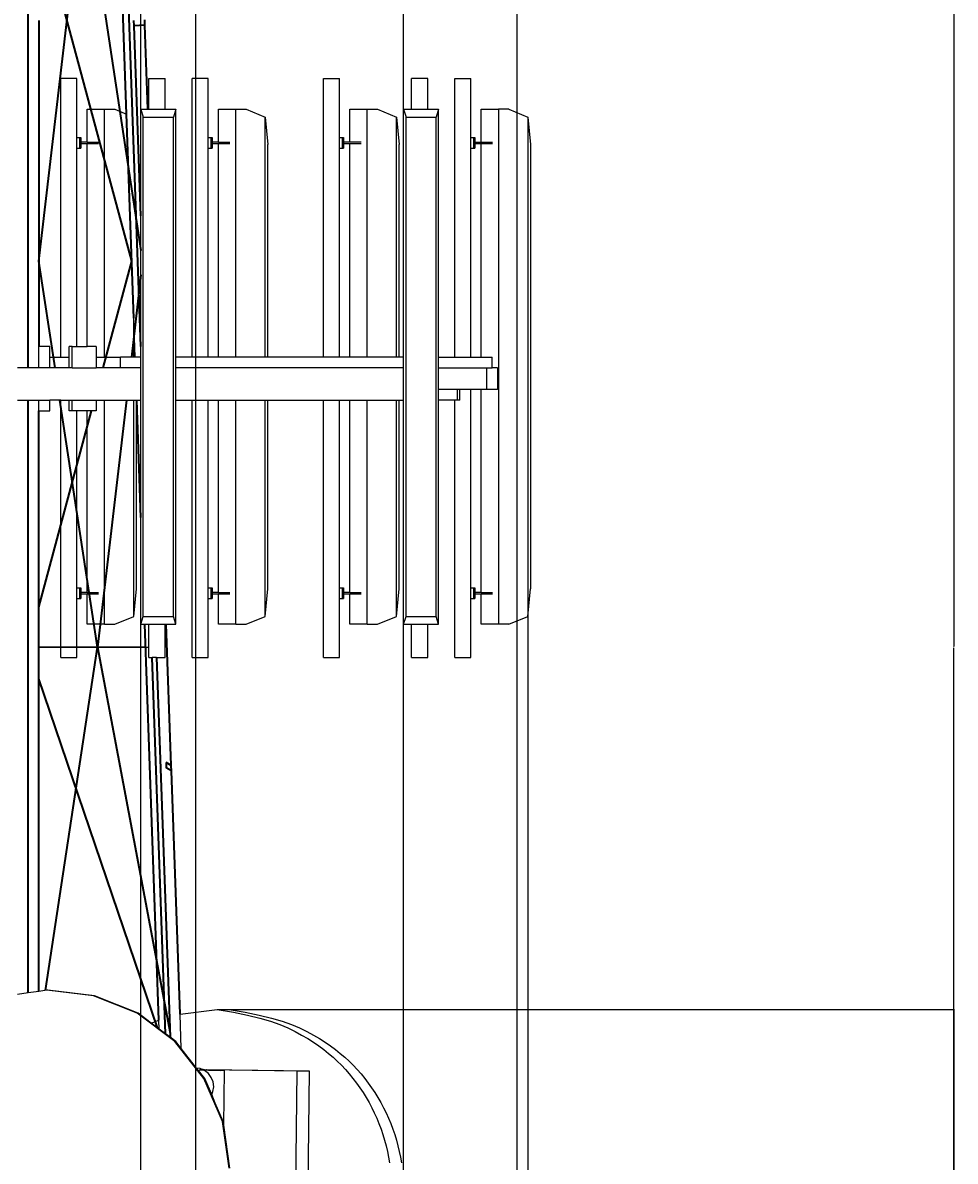
# Model space of a CAD drawing. Units: inches. Extents: x 3780 to 4301, y 1637 to 4224.
# Tile 7 of 8: x 4040 to 4301, y 3542 to 3860. Entities that reach past the tile are written whole.
import ezdxf

# ---------------------------------------------------------------- set-up
doc = ezdxf.new("R2010")
doc.units = ezdxf.units.IN
for name, color, linetype, lineweight in [('A-ANNO-DIMS', 2, 'Continuous', 18), ('E-COMM-ANTN', 4, 'Continuous', 25), ('E-COMM-DISH', 3, 'Continuous', 25), ('S-TOWR', 7, 'Continuous', 35)]:
    doc.layers.add(name, color=color, linetype=linetype, lineweight=lineweight)
doc.styles.get("Standard").update_dxf_attribs({"font": 'arial.ttf'})
doc.dimstyles.get("Standard").update_dxf_attribs({"dimtxt": 0.18, "dimasz": 0.18, "dimexe": 0.18, "dimexo": 0.0625, "dimgap": 0.09, "dimtad": 0, "dimtih": 1, "dimtoh": 1, "dimdec": 4, "dimzin": 0, "dimdsep": 46, "dimtxsty": 'Standard', "dimcen": 0.09, "dimadec": 0, "dimazin": 0, "dimtfac": 1, "dimtdec": 4, "dimtofl": 0, "dimtmove": 0, "dimatfit": 3, "dimfxl": 1, "dimtolj": 1, "dimtzin": 0, "dimarcsym": 0})

# ---------------------------------------------------------------- blocks, each defined once
blk = doc.blocks.new('ANT-PANEL')
for p, q in [((3905.38, 3835.91), (3900.05, 3833.75)), ((3905.38, 3835.91), (3908.22, 3835.91)), ((3908.22, 3691.91), (3908.22, 3835.91)), ((3900.05, 3833.75), (3899.34, 3826.07)), ((3900.05, 3694.07), (3900.05, 3833.75)), ((3899.34, 3701.75), (3899.34, 3826.07)), ((3900.05, 3694.07), (3899.34, 3701.75)), ((3905.38, 3691.91), (3900.05, 3694.07)), ((3905.38, 3691.91), (3908.22, 3691.91))]:
    blk.add_line(p, q)
blk = doc.blocks.new('ANT-PANEL-MOUNT-B')
for p, q in [((4148.97, 3835.91), (4148.97, 3844.56)), ((4153.47, 3844.56), (4148.97, 3844.56)), ((4153.47, 3835.91), (4153.47, 3844.56)), ((4146.73, 3835.91), (4147.4, 3833.75)), ((4146.73, 3835.91), (4148.97, 3835.91)), ((4146.73, 3766.56), (4146.73, 3835.91)), ((4148.97, 3835.91), (4153.47, 3835.91)), ((4153.47, 3835.91), (4156.48, 3835.91)), ((4156.48, 3835.91), (4155.82, 3833.75)), ((4156.48, 3766.56), (4156.48, 3835.91)), ((4147.4, 3833.75), (4155.82, 3833.75)), ((4147.4, 3694.07), (4147.4, 3833.75)), ((4155.82, 3694.07), (4155.82, 3833.75)), ((4146.73, 3763.56), (4146.73, 3766.56)), ((4156.48, 3763.56), (4156.48, 3766.56)), ((4146.73, 3754.56), (4146.73, 3763.56)), ((4156.48, 3757.56), (4156.48, 3763.56)), ((4156.48, 3754.56), (4156.48, 3757.56)), ((4146.73, 3691.91), (4146.73, 3754.56)), ((4156.48, 3691.91), (4156.48, 3754.56)), ((4146.73, 3691.91), (4147.4, 3694.07)), ((4146.73, 3691.91), (4148.97, 3691.91)), ((4147.4, 3694.07), (4155.82, 3694.07)), ((4148.97, 3682.56), (4148.97, 3691.91)), ((4148.97, 3691.91), (4153.47, 3691.91)), ((4153.47, 3682.56), (4153.47, 3691.91)), ((4153.47, 3691.91), (4156.48, 3691.91)), ((4156.48, 3691.91), (4155.82, 3694.07)), ((4148.97, 3682.56), (4153.47, 3682.56))]:
    blk.add_line(p, q)
blk = doc.blocks.new('*D21')
at = {"layer": 'A-ANNO-DIMS', "color": 0, "lineweight": -2, "transparency": 16777216}
for p, q in [((4010.55, 3901.46), (4300.89, 3901.46)), ((4300.71, 3901.28), (4300.71, 3685.65)), ((4300.71, 3469.64), (4300.71, 3685.28)), ((4044.72, 3469.46), (4300.89, 3469.46))]:
    blk.add_line(p, q, dxfattribs=at)
at = {"layer": 'A-ANNO-DIMS', "color": 0, "transparency": 16777216}
for points in [[(4300.68, 3901.28), (4300.74, 3901.28), (4300.71, 3901.46)], [(4300.68, 3469.64), (4300.74, 3469.64), (4300.71, 3469.46)]]:
    blk.add_solid(points, dxfattribs=at)
at = {"layer": 'Defpoints', "color": 0, "transparency": 16777216}
for p in [(4010.49, 3901.46), (4300.71, 3901.46), (4044.66, 3469.46)]:
    blk.add_point(p, dxfattribs=at)
at = {"layer": 'A-ANNO-DIMS', "color": 0, "transparency": 16777216, "insert": (4300.71, 3685.46), "char_height": 0.18, "attachment_point": 5}
blk.add_mtext('\\A1;432', dxfattribs=at)
blk = doc.blocks.new('*D22')
at = {"layer": 'A-ANNO-DIMS', "color": 0, "lineweight": -2, "transparency": 16777216}
for p, q in [((3900.05, 3694.01), (3900.05, 1636.57)), ((4181.5, 3694.01), (4181.5, 1636.57)), ((3900.23, 1636.75), (4040.31, 1636.75)), ((4181.32, 1636.75), (4041.24, 1636.75))]:
    blk.add_line(p, q, dxfattribs=at)
at = {"layer": 'A-ANNO-DIMS', "color": 0, "transparency": 16777216}
for points in [[(3900.23, 1636.78), (3900.23, 1636.72), (3900.05, 1636.75)], [(4181.32, 1636.78), (4181.32, 1636.72), (4181.5, 1636.75)]]:
    blk.add_solid(points, dxfattribs=at)
at = {"layer": 'Defpoints', "color": 0, "transparency": 16777216}
for p in [(3900.05, 3694.07), (4181.5, 3694.07), (4181.5, 1636.75)]:
    blk.add_point(p, dxfattribs=at)
at = {"layer": 'A-ANNO-DIMS', "color": 0, "transparency": 16777216, "insert": (4040.77, 1636.75), "char_height": 0.18, "attachment_point": 5}
blk.add_mtext('\\A1;281.45', dxfattribs=at)
blk = doc.blocks.new('*D28')
at = {"layer": 'A-ANNO-DIMS', "color": 0, "lineweight": -2, "transparency": 16777216}
for p, q in [((3926.17, 3691.91), (3780.66, 3691.91)), ((3780.84, 3691.73), (3780.84, 3590.48)), ((3780.84, 3488.87), (3780.84, 3590.12)), ((4048.31, 3488.69), (3780.66, 3488.69))]:
    blk.add_line(p, q, dxfattribs=at)
at = {"layer": 'A-ANNO-DIMS', "color": 0, "transparency": 16777216}
for points in [[(3780.81, 3691.73), (3780.87, 3691.73), (3780.84, 3691.91)], [(3780.81, 3488.87), (3780.87, 3488.87), (3780.84, 3488.69)]]:
    blk.add_solid(points, dxfattribs=at)
at = {"layer": 'Defpoints', "color": 0, "transparency": 16777216}
for p in [(3780.84, 3691.91), (3926.23, 3691.91), (4048.37, 3488.69)]:
    blk.add_point(p, dxfattribs=at)
at = {"layer": 'A-ANNO-DIMS', "color": 0, "transparency": 16777216, "insert": (3780.84, 3590.3), "char_height": 0.18, "attachment_point": 5}
blk.add_mtext('\\A1;203.2', dxfattribs=at)
blk = doc.blocks.new('*D40')
at = {"layer": 'A-ANNO-DIMS', "color": 0, "lineweight": -2, "transparency": 16777216}
for p, q in [((3999.73, 3835.97), (3999.73, 4223.96)), ((3999.91, 4223.78), (4036.16, 4223.78)), ((4073.05, 4223.78), (4036.81, 4223.78)), ((4073.23, 3835.97), (4073.23, 4223.96))]:
    blk.add_line(p, q, dxfattribs=at)
at = {"layer": 'A-ANNO-DIMS', "color": 0, "transparency": 16777216}
for points in [[(3999.91, 4223.81), (3999.91, 4223.75), (3999.73, 4223.78)], [(4073.05, 4223.81), (4073.05, 4223.75), (4073.23, 4223.78)]]:
    blk.add_solid(points, dxfattribs=at)
at = {"layer": 'Defpoints', "color": 0, "transparency": 16777216}
for p in [(4073.23, 4223.78), (3999.73, 3835.91), (4073.23, 3835.91)]:
    blk.add_point(p, dxfattribs=at)
at = {"layer": 'A-ANNO-DIMS', "color": 0, "transparency": 16777216, "insert": (4036.48, 4223.78), "char_height": 0.18, "attachment_point": 5}
blk.add_mtext('\\A1;73.5', dxfattribs=at)
blk = doc.blocks.new('*D41')
at = {"layer": 'A-ANNO-DIMS', "color": 0, "lineweight": -2, "transparency": 16777216}
for p, q in [((4073.23, 3835.97), (4073.23, 4223.96)), ((4073.41, 4223.78), (4109.66, 4223.78)), ((4146.55, 4223.78), (4110.31, 4223.78)), ((4146.73, 3835.97), (4146.73, 4223.96))]:
    blk.add_line(p, q, dxfattribs=at)
at = {"layer": 'A-ANNO-DIMS', "color": 0, "transparency": 16777216}
for points in [[(4073.41, 4223.81), (4073.41, 4223.75), (4073.23, 4223.78)], [(4146.55, 4223.81), (4146.55, 4223.75), (4146.73, 4223.78)]]:
    blk.add_solid(points, dxfattribs=at)
at = {"layer": 'Defpoints', "color": 0, "transparency": 16777216}
for p in [(4146.73, 4223.78), (4073.23, 3835.91), (4146.73, 3835.91)]:
    blk.add_point(p, dxfattribs=at)
at = {"layer": 'A-ANNO-DIMS', "color": 0, "transparency": 16777216, "insert": (4109.98, 4223.78), "char_height": 0.18, "attachment_point": 5}
blk.add_mtext('\\A1;73.5', dxfattribs=at)
blk = doc.blocks.new('*D45')
at = {"layer": 'A-ANNO-DIMS', "color": 0, "lineweight": -2, "transparency": 16777216}
for p, q in [((3971.79, 3552.9), (3780.66, 3552.9)), ((3780.84, 3552.72), (3780.84, 3520.98)), ((3780.84, 3488.87), (3780.84, 3520.61)), ((4048.31, 3488.69), (3780.66, 3488.69))]:
    blk.add_line(p, q, dxfattribs=at)
at = {"layer": 'A-ANNO-DIMS', "color": 0, "transparency": 16777216}
for points in [[(3780.81, 3552.72), (3780.87, 3552.72), (3780.84, 3552.9)], [(3780.81, 3488.87), (3780.87, 3488.87), (3780.84, 3488.69)]]:
    blk.add_solid(points, dxfattribs=at)
at = {"layer": 'Defpoints', "color": 0, "transparency": 16777216}
for p in [(3780.84, 3552.9), (3971.85, 3552.9), (4048.37, 3488.69)]:
    blk.add_point(p, dxfattribs=at)
at = {"layer": 'A-ANNO-DIMS', "color": 0, "transparency": 16777216, "insert": (3780.84, 3520.8), "char_height": 0.18, "attachment_point": 5}
blk.add_mtext('\\A1;64.21', dxfattribs=at)
blk = doc.blocks.new('*D47')
at = {"layer": 'A-ANNO-DIMS', "color": 0, "lineweight": -2, "transparency": 16777216}
for p, q in [((4094.64, 3584.08), (4300.89, 3584.08)), ((4300.71, 3583.9), (4300.71, 3533.86)), ((4300.71, 3483.47), (4300.71, 3533.5)), ((4093.42, 3483.29), (4300.89, 3483.29))]:
    blk.add_line(p, q, dxfattribs=at)
at = {"layer": 'A-ANNO-DIMS', "color": 0, "transparency": 16777216}
for points in [[(4300.68, 3583.9), (4300.74, 3583.9), (4300.71, 3584.08)], [(4300.68, 3483.47), (4300.74, 3483.47), (4300.71, 3483.29)]]:
    blk.add_solid(points, dxfattribs=at)
at = {"layer": 'Defpoints', "color": 0, "transparency": 16777216}
for p in [(4094.58, 3584.08), (4093.36, 3483.29), (4300.71, 3483.29)]:
    blk.add_point(p, dxfattribs=at)
at = {"layer": 'A-ANNO-DIMS', "color": 0, "transparency": 16777216, "insert": (4300.71, 3533.68), "char_height": 0.18, "attachment_point": 5}
blk.add_mtext('\\A1;100.79', dxfattribs=at)
blk = doc.blocks.new('*D49')
at = {"layer": 'A-ANNO-DIMS', "color": 0, "lineweight": -2, "transparency": 16777216}
for p, q in [((3999.73, 3245.63), (3999.73, 4223.96)), ((3999.91, 4223.78), (4036.16, 4223.78)), ((4073.05, 4223.78), (4036.81, 4223.78)), ((4073.23, 3245.63), (4073.23, 4223.96))]:
    blk.add_line(p, q, dxfattribs=at)
at = {"layer": 'A-ANNO-DIMS', "color": 0, "transparency": 16777216}
for points in [[(3999.91, 4223.81), (3999.91, 4223.75), (3999.73, 4223.78)], [(4073.05, 4223.81), (4073.05, 4223.75), (4073.23, 4223.78)]]:
    blk.add_solid(points, dxfattribs=at)
at = {"layer": 'Defpoints', "color": 0, "transparency": 16777216}
for p in [(4073.23, 4223.78), (3999.73, 3245.56), (4073.23, 3245.56)]:
    blk.add_point(p, dxfattribs=at)
at = {"layer": 'A-ANNO-DIMS', "color": 0, "transparency": 16777216, "insert": (4036.48, 4223.78), "char_height": 0.18, "attachment_point": 5}
blk.add_mtext('\\A1;73.5', dxfattribs=at)
blk = doc.blocks.new('*D50')
at = {"layer": 'A-ANNO-DIMS', "color": 0, "lineweight": -2, "transparency": 16777216}
for p, q in [((4073.23, 3245.63), (4073.23, 4223.96)), ((4073.41, 4223.78), (4109.66, 4223.78)), ((4146.55, 4223.78), (4110.31, 4223.78)), ((4146.73, 3245.63), (4146.73, 4223.96))]:
    blk.add_line(p, q, dxfattribs=at)
at = {"layer": 'A-ANNO-DIMS', "color": 0, "transparency": 16777216}
for points in [[(4073.41, 4223.81), (4073.41, 4223.75), (4073.23, 4223.78)], [(4146.55, 4223.81), (4146.55, 4223.75), (4146.73, 4223.78)]]:
    blk.add_solid(points, dxfattribs=at)
at = {"layer": 'Defpoints', "color": 0, "transparency": 16777216}
for p in [(4146.73, 4223.78), (4073.23, 3245.56), (4146.73, 3245.56)]:
    blk.add_point(p, dxfattribs=at)
at = {"layer": 'A-ANNO-DIMS', "color": 0, "transparency": 16777216, "insert": (4109.98, 4223.78), "char_height": 0.18, "attachment_point": 5}
blk.add_mtext('\\A1;73.5', dxfattribs=at)
blk = doc.blocks.new('*D59')
at = {"layer": 'A-ANNO-DIMS', "color": 0, "lineweight": -2, "transparency": 16777216}
for p, q in [((4088.55, 3352.58), (4088.55, 4223.96)), ((4088.73, 4223.78), (4133.13, 4223.78)), ((4178.28, 4223.78), (4133.88, 4223.78)), ((4178.46, 3329.55), (4178.46, 4223.96))]:
    blk.add_line(p, q, dxfattribs=at)
at = {"layer": 'A-ANNO-DIMS', "color": 0, "transparency": 16777216}
for points in [[(4088.73, 4223.81), (4088.73, 4223.75), (4088.55, 4223.78)], [(4178.28, 4223.81), (4178.28, 4223.75), (4178.46, 4223.78)]]:
    blk.add_solid(points, dxfattribs=at)
at = {"layer": 'Defpoints', "color": 0, "transparency": 16777216}
for p in [(4178.46, 4223.78), (4088.55, 3352.51), (4178.46, 3329.49)]:
    blk.add_point(p, dxfattribs=at)
at = {"layer": 'A-ANNO-DIMS', "color": 0, "transparency": 16777216, "insert": (4133.51, 4223.78), "char_height": 0.18, "attachment_point": 5}
blk.add_mtext('\\A1;89.91', dxfattribs=at)

msp = doc.modelspace()

# ---------------------------------------------------------------- linework, layer by layer
at = {"layer": 'E-COMM-ANTN'}
for p, q in [((4050.7911, 3766.5582), (4050.7911, 3844.5582)), ((4055.2911, 3844.5582), (4050.7911, 3844.5582)), ((4055.2911, 3828.0582), (4055.2911, 3844.5582)), ((4075.4676, 3835.9077), (4075.4676, 3844.5582)), ((4075.4676, 3844.5582), (4079.9676, 3844.5582)), ((4079.9676, 3835.9077), (4079.9676, 3844.5582)), ((4087.5411, 3766.5582), (4087.5411, 3844.5582)), ((4092.0411, 3844.5582), (4087.5411, 3844.5582)), ((4092.0411, 3828.0582), (4092.0411, 3844.5582)), ((4124.2911, 3766.5582), (4124.2911, 3844.5582)), ((4124.2911, 3844.5582), (4128.7911, 3844.5582)), ((4128.7911, 3828.0582), (4128.7911, 3844.5582)), ((4161.0411, 3766.5582), (4161.0411, 3844.5582)), ((4161.0411, 3844.5582), (4165.5411, 3844.5582)), ((4165.5411, 3828.0582), (4165.5411, 3844.5582)), ((4058.2034, 3826.7457), (4058.2034, 3835.9077)), ((4058.2034, 3835.9077), (4063.0784, 3835.9077)), ((4063.0784, 3835.9077), (4065.9127, 3835.9077)), ((4063.0784, 3766.5582), (4063.0784, 3835.9077)), ((4065.9127, 3835.9077), (4069.2183, 3834.5694)), ((4073.2315, 3835.9077), (4073.8979, 3833.7477)), ((4073.2315, 3835.9077), (4075.1707, 3835.9077)), ((4073.2315, 3806.0827), (4073.2315, 3835.9077)), ((4075.1707, 3835.9077), (4075.4676, 3835.9077)), ((4075.4676, 3835.9077), (4079.9676, 3835.9077)), ((4079.9676, 3835.9077), (4082.9815, 3835.9077)), ((4082.9815, 3835.9077), (4082.3151, 3833.7477)), ((4082.9815, 3766.5582), (4082.9815, 3835.9077)), ((4094.9534, 3826.7457), (4094.9534, 3835.9077)), ((4094.9534, 3835.9077), (4099.8284, 3835.9077)), ((4099.8284, 3835.9077), (4102.6627, 3835.9077)), ((4099.8284, 3766.5582), (4099.8284, 3835.9077)), ((4102.6627, 3835.9077), (4107.998, 3833.7477)), ((4131.7034, 3826.7457), (4131.7034, 3835.9077)), ((4131.7034, 3835.9077), (4136.5784, 3835.9077)), ((4136.5784, 3835.9077), (4139.4127, 3835.9077)), ((4136.5784, 3766.5582), (4136.5784, 3835.9077)), ((4139.4127, 3835.9077), (4144.748, 3833.7477)), ((4168.4534, 3826.7457), (4168.4534, 3835.9077)), ((4168.4534, 3835.9077), (4173.3284, 3835.9077)), ((4073.8979, 3833.7477), (4082.3151, 3833.7477)), ((4073.8979, 3694.0677), (4073.8979, 3833.7477)), ((4082.3151, 3694.0677), (4082.3151, 3833.7477)), ((4107.998, 3766.5582), (4107.998, 3833.7477)), ((4107.998, 3833.7477), (4108.7091, 3826.0653)), ((4144.748, 3833.7477), (4145.4591, 3826.0653)), ((4144.748, 3766.5582), (4144.748, 3833.7477)), ((4055.2911, 3828.0582), (4056.1147, 3828.0582)), ((4055.2911, 3825.0582), (4055.2911, 3828.0582)), ((4056.1147, 3828.0582), (4056.4394, 3828.0582)), ((4056.1147, 3825.0582), (4056.1147, 3828.0582)), ((4056.4394, 3828.0582), (4056.4394, 3826.7457)), ((4092.0411, 3828.0582), (4092.8647, 3828.0582)), ((4092.0411, 3825.0582), (4092.0411, 3828.0582)), ((4092.8647, 3828.0582), (4093.1894, 3828.0582)), ((4092.8647, 3825.0582), (4092.8647, 3828.0582)), ((4093.1894, 3828.0582), (4093.1894, 3826.7457)), ((4128.7911, 3828.0582), (4129.6147, 3828.0582)), ((4128.7911, 3825.0582), (4128.7911, 3828.0582)), ((4129.6147, 3825.0582), (4129.6147, 3828.0582)), ((4129.6147, 3828.0582), (4129.9394, 3828.0582)), ((4129.9394, 3828.0582), (4129.9394, 3826.7457)), ((4165.5411, 3828.0582), (4166.3647, 3828.0582)), ((4165.5411, 3825.0582), (4165.5411, 3828.0582)), ((4166.3647, 3828.0582), (4166.6894, 3828.0582)), ((4166.3647, 3825.0582), (4166.3647, 3828.0582)), ((4166.6894, 3828.0582), (4166.6894, 3826.7457)), ((4055.2911, 3825.0582), (4056.1147, 3825.0582)), ((4055.2911, 3769.5582), (4055.2911, 3825.0582)), ((4056.1147, 3825.0582), (4056.4394, 3825.0582)), ((4058.2034, 3826.7457), (4056.4394, 3826.7457)), ((4056.4394, 3826.7457), (4056.4394, 3826.3707)), ((4056.4394, 3826.3707), (4056.4394, 3825.0582)), ((4056.4394, 3826.3707), (4058.2034, 3826.3707)), ((4058.2034, 3826.7457), (4061.3979, 3826.7457)), ((4058.2034, 3769.5582), (4058.2034, 3826.3707)), ((4058.2034, 3826.3707), (4061.3979, 3826.3707)), ((4092.0411, 3825.0582), (4092.8647, 3825.0582)), ((4092.0411, 3766.5582), (4092.0411, 3825.0582)), ((4092.8647, 3825.0582), (4093.1894, 3825.0582)), ((4094.9534, 3826.7457), (4093.1894, 3826.7457)), ((4093.1894, 3826.7457), (4093.1894, 3826.3707)), ((4093.1894, 3826.3707), (4094.9534, 3826.3707)), ((4093.1894, 3826.3707), (4093.1894, 3825.0582)), ((4094.9534, 3826.7457), (4098.1479, 3826.7457)), ((4094.9534, 3766.5582), (4094.9534, 3826.3707)), ((4094.9534, 3826.3707), (4098.1479, 3826.3707)), ((4108.7091, 3766.5582), (4108.7091, 3826.0653)), ((4128.7911, 3825.0582), (4129.6147, 3825.0582)), ((4128.7911, 3766.5582), (4128.7911, 3825.0582)), ((4129.6147, 3825.0582), (4129.9394, 3825.0582)), ((4131.7034, 3826.7457), (4129.9394, 3826.7457)), ((4129.9394, 3826.7457), (4129.9394, 3826.3707)), ((4129.9394, 3826.3707), (4131.7034, 3826.3707)), ((4129.9394, 3826.3707), (4129.9394, 3825.0582)), ((4134.8979, 3826.7457), (4131.7034, 3826.7457)), ((4131.7034, 3766.5582), (4131.7034, 3826.3707)), ((4131.7034, 3826.3707), (4134.8979, 3826.3707)), ((4145.4591, 3766.5582), (4145.4591, 3826.0653)), ((4165.5411, 3825.0582), (4166.3647, 3825.0582)), ((4165.5411, 3766.5582), (4165.5411, 3825.0582)), ((4166.3647, 3825.0582), (4166.6894, 3825.0582)), ((4166.6894, 3826.7457), (4168.4534, 3826.7457)), ((4166.6894, 3826.7457), (4166.6894, 3826.3707)), ((4166.6894, 3826.3707), (4168.4534, 3826.3707)), ((4166.6894, 3826.3707), (4166.6894, 3825.0582)), ((4168.4534, 3826.7457), (4171.6479, 3826.7457)), ((4168.4534, 3766.5582), (4168.4534, 3826.3707)), ((4168.4534, 3826.3707), (4171.6479, 3826.3707)), ((4073.2315, 3769.5583), (4073.2315, 3806.0827)), ((4071.248, 3766.5582), (4071.248, 3777.502)), ((4071.6372, 3766.5582), (4071.248, 3777.502)), ((4047.7176, 3769.5582), (4044.6622, 3769.5582)), ((4044.6622, 3763.5582), (4044.6622, 3769.5582)), ((4047.7176, 3766.5582), (4047.7176, 3769.5582)), ((4053.9472, 3769.5582), (4053.181, 3769.5582)), ((4053.181, 3766.5582), (4053.181, 3769.5582)), ((4053.9472, 3763.5582), (4053.9472, 3769.5582)), ((4053.9472, 3769.5582), (4055.2911, 3769.5582)), ((4055.2911, 3769.5582), (4058.2034, 3769.5582)), ((4060.6972, 3769.5582), (4058.2034, 3769.5582)), ((4060.6972, 3769.5582), (4060.6972, 3766.5582)), ((4073.2315, 3766.5582), (4073.2315, 3769.5583)), ((4047.7176, 3763.5582), (4047.7176, 3766.5582)), ((4047.7176, 3766.5582), (4050.7911, 3766.5582)), ((4050.7911, 3766.5582), (4053.181, 3766.5582)), ((4053.181, 3763.5582), (4053.181, 3766.5582)), ((4060.6972, 3766.5582), (4060.6972, 3763.5582)), ((4060.6972, 3766.5582), (4063.0784, 3766.5582)), ((4063.0784, 3766.5582), (4067.5445, 3766.5582)), ((4067.5445, 3763.5582), (4067.5445, 3766.5582)), ((4071.248, 3766.5582), (4067.5445, 3766.5582)), ((4071.6372, 3766.5582), (4071.248, 3766.5582)), ((4073.2315, 3766.5582), (4071.6372, 3766.5582)), ((4073.2315, 3763.5582), (4073.2315, 3766.5582)), ((4087.5411, 3766.5582), (4082.9815, 3766.5582)), ((4082.9815, 3763.5582), (4082.9815, 3766.5582)), ((4092.0411, 3766.5582), (4087.5411, 3766.5582)), ((4094.9534, 3766.5582), (4092.0411, 3766.5582)), ((4099.8284, 3766.5582), (4094.9534, 3766.5582)), ((4107.998, 3766.5582), (4099.8284, 3766.5582)), ((4108.7091, 3766.5582), (4107.998, 3766.5582)), ((4124.2911, 3766.5582), (4108.7091, 3766.5582)), ((4128.7911, 3766.5582), (4124.2911, 3766.5582)), ((4131.7034, 3766.5582), (4128.7911, 3766.5582)), ((4136.5784, 3766.5582), (4131.7034, 3766.5582)), ((4144.748, 3766.5582), (4136.5784, 3766.5582)), ((4145.4591, 3766.5582), (4144.748, 3766.5582)), ((4146.7315, 3766.5582), (4145.4591, 3766.5582)), ((4156.4815, 3766.5582), (4161.0411, 3766.5582)), ((4161.0411, 3766.5582), (4165.5411, 3766.5582)), ((4165.5411, 3766.5582), (4168.4534, 3766.5582)), ((4168.4534, 3766.5582), (4171.4676, 3766.5582)), ((4171.4676, 3763.5582), (4171.4676, 3766.5582)), ((4041.6622, 3763.5582), (4038.6622, 3763.5582)), ((4044.6622, 3763.5582), (4041.6622, 3763.5582)), ((4047.7176, 3763.5582), (4044.6622, 3763.5582)), ((4053.181, 3763.5582), (4047.7176, 3763.5582)), ((4053.9472, 3763.5582), (4053.181, 3763.5582)), ((4053.9472, 3763.5582), (4060.6972, 3763.5582)), ((4067.5445, 3763.5582), (4060.6972, 3763.5582)), ((4073.2315, 3763.5582), (4067.5445, 3763.5582)), ((4073.2315, 3754.5582), (4073.2315, 3763.5582)), ((4146.7315, 3763.5582), (4082.9815, 3763.5582)), ((4082.9815, 3754.5582), (4082.9815, 3763.5582)), ((4156.4815, 3763.5582), (4169.976, 3763.5582)), ((4169.976, 3763.5582), (4171.4676, 3763.5582)), ((4169.976, 3757.5582), (4169.976, 3763.5582)), ((4172.9591, 3763.5582), (4171.4676, 3763.5582)), ((4172.9591, 3763.5582), (4172.9591, 3757.5582)), ((4161.818, 3757.5582), (4156.4815, 3757.5582)), ((4161.818, 3754.5582), (4161.818, 3757.5582)), ((4162.4676, 3757.5582), (4161.818, 3757.5582)), ((4162.4676, 3754.5582), (4162.4676, 3757.5582)), ((4165.5411, 3757.5582), (4162.4676, 3757.5582)), ((4165.5411, 3702.0582), (4165.5411, 3757.5582)), ((4168.4534, 3757.5582), (4165.5411, 3757.5582)), ((4168.4534, 3700.7457), (4168.4534, 3757.5582)), ((4169.976, 3757.5582), (4168.4534, 3757.5582)), ((4172.9591, 3757.5582), (4169.976, 3757.5582)), ((4038.6622, 3754.5582), (4041.6622, 3754.5582)), ((4041.6622, 3754.5582), (4044.6622, 3754.5582)), ((4044.6622, 3751.5582), (4044.6622, 3754.5582)), ((4044.6622, 3754.5582), (4047.7176, 3754.5582)), ((4044.6622, 3751.5582), (4047.7176, 3751.5582)), ((4047.7176, 3751.5582), (4047.7176, 3754.5582)), ((4050.7911, 3754.5582), (4047.7176, 3754.5582)), ((4050.7911, 3682.5582), (4050.7911, 3754.5582)), ((4050.7911, 3754.5582), (4053.181, 3754.5582)), ((4053.181, 3751.5582), (4053.181, 3754.5582)), ((4053.181, 3754.5582), (4053.9472, 3754.5582)), ((4053.9472, 3751.5582), (4053.181, 3751.5582)), ((4053.9472, 3751.5582), (4053.9472, 3754.5582)), ((4053.9472, 3754.5582), (4060.6972, 3754.5582)), ((4055.2911, 3751.5582), (4053.9472, 3751.5582)), ((4058.2034, 3751.5582), (4055.2911, 3751.5582)), ((4055.2911, 3702.0582), (4055.2911, 3751.5582)), ((4058.2034, 3700.7457), (4058.2034, 3751.5582)), ((4060.6972, 3751.5582), (4058.2034, 3751.5582)), ((4060.6972, 3754.5582), (4060.6972, 3751.5582)), ((4060.6972, 3754.5582), (4063.0784, 3754.5582)), ((4063.0784, 3691.9077), (4063.0784, 3754.5582)), ((4063.0784, 3754.5582), (4071.248, 3754.5582)), ((4071.248, 3694.0677), (4071.248, 3754.5582)), ((4071.248, 3754.5582), (4071.9591, 3754.5582)), ((4071.9591, 3701.7501), (4071.9591, 3754.5582)), ((4071.9591, 3754.5582), (4072.064, 3754.5582)), ((4072.064, 3754.5582), (4073.2315, 3754.5582)), ((4073.2315, 3721.7331), (4073.2315, 3754.5582)), ((4082.9815, 3691.9077), (4082.9815, 3754.5582)), ((4082.9815, 3754.5582), (4087.5411, 3754.5582)), ((4087.5411, 3682.5582), (4087.5411, 3754.5582)), ((4087.5411, 3754.5582), (4092.0411, 3754.5582)), ((4092.0411, 3754.5582), (4094.9534, 3754.5582)), ((4092.0411, 3702.0582), (4092.0411, 3754.5582)), ((4094.9534, 3700.7457), (4094.9534, 3754.5582)), ((4094.9534, 3754.5582), (4099.8284, 3754.5582)), ((4099.8284, 3691.9077), (4099.8284, 3754.5582)), ((4099.8284, 3754.5582), (4107.998, 3754.5582)), ((4107.998, 3694.0677), (4107.998, 3754.5582)), ((4107.998, 3754.5582), (4108.7091, 3754.5582)), ((4108.7091, 3701.7501), (4108.7091, 3754.5582)), ((4108.7091, 3754.5582), (4124.2911, 3754.5582)), ((4124.2911, 3682.5582), (4124.2911, 3754.5582)), ((4124.2911, 3754.5582), (4128.7911, 3754.5582)), ((4128.7911, 3702.0582), (4128.7911, 3754.5582)), ((4128.7911, 3754.5582), (4131.7034, 3754.5582)), ((4131.7034, 3700.7457), (4131.7034, 3754.5582)), ((4131.7034, 3754.5582), (4136.5784, 3754.5582)), ((4136.5784, 3691.9077), (4136.5784, 3754.5582)), ((4136.5784, 3754.5582), (4144.748, 3754.5582)), ((4144.748, 3694.0677), (4144.748, 3754.5582)), ((4144.748, 3754.5582), (4145.4591, 3754.5582)), ((4145.4591, 3701.7501), (4145.4591, 3754.5582)), ((4145.4591, 3754.5582), (4146.7315, 3754.5582)), ((4161.0411, 3754.5582), (4156.4815, 3754.5582)), ((4161.0411, 3682.5582), (4161.0411, 3754.5582)), ((4161.818, 3754.5582), (4161.0411, 3754.5582)), ((4162.4676, 3754.5582), (4161.818, 3754.5582)), ((4073.2315, 3691.9077), (4073.2315, 3721.7331)), ((4055.2911, 3702.0582), (4056.1147, 3702.0582)), ((4055.2911, 3699.0582), (4055.2911, 3702.0582)), ((4056.1147, 3699.0582), (4056.1147, 3702.0582)), ((4056.1147, 3702.0582), (4056.4394, 3702.0582)), ((4056.4394, 3702.0582), (4056.4394, 3700.7457)), ((4058.2034, 3700.7457), (4056.4394, 3700.7457)), ((4056.4394, 3700.7457), (4056.4394, 3700.3707)), ((4058.2034, 3700.7457), (4061.3979, 3700.7457)), ((4071.248, 3694.0677), (4071.9591, 3701.7501)), ((4092.0411, 3702.0582), (4092.8647, 3702.0582)), ((4092.0411, 3699.0582), (4092.0411, 3702.0582)), ((4092.8647, 3702.0582), (4093.1894, 3702.0582)), ((4092.8647, 3699.0582), (4092.8647, 3702.0582)), ((4093.1894, 3702.0582), (4093.1894, 3700.7457)), ((4094.9534, 3700.7457), (4093.1894, 3700.7457)), ((4093.1894, 3700.7457), (4093.1894, 3700.3707)), ((4094.9534, 3700.7457), (4098.1479, 3700.7457)), ((4107.998, 3694.0677), (4108.7091, 3701.7501)), ((4128.7911, 3702.0582), (4129.6147, 3702.0582)), ((4128.7911, 3699.0582), (4128.7911, 3702.0582)), ((4129.6147, 3699.0582), (4129.6147, 3702.0582)), ((4129.6147, 3702.0582), (4129.9394, 3702.0582)), ((4129.9394, 3702.0582), (4129.9394, 3700.7457)), ((4131.7034, 3700.7457), (4129.9394, 3700.7457)), ((4129.9394, 3700.7457), (4129.9394, 3700.3707)), ((4131.7034, 3700.7457), (4134.8979, 3700.7457)), ((4144.748, 3694.0677), (4145.4591, 3701.7501)), ((4165.5411, 3702.0582), (4166.3647, 3702.0582)), ((4165.5411, 3699.0582), (4165.5411, 3702.0582)), ((4166.3647, 3702.0582), (4166.6894, 3702.0582)), ((4166.3647, 3699.0582), (4166.3647, 3702.0582)), ((4166.6894, 3702.0582), (4166.6894, 3700.7457)), ((4168.4534, 3700.7457), (4166.6894, 3700.7457)), ((4166.6894, 3700.7457), (4166.6894, 3700.3707)), ((4168.4534, 3700.7457), (4171.6479, 3700.7457)), ((4055.2911, 3699.0582), (4056.1147, 3699.0582)), ((4055.2911, 3682.5582), (4055.2911, 3699.0582)), ((4056.1147, 3699.0582), (4056.4394, 3699.0582)), ((4056.4394, 3700.3707), (4056.4394, 3699.0582)), ((4056.4394, 3700.3707), (4058.2034, 3700.3707)), ((4058.2034, 3691.9077), (4058.2034, 3700.3707)), ((4058.2034, 3700.3707), (4061.3979, 3700.3707)), ((4092.0411, 3699.0582), (4092.8647, 3699.0582)), ((4092.0411, 3682.5582), (4092.0411, 3699.0582)), ((4092.8647, 3699.0582), (4093.1894, 3699.0582)), ((4093.1894, 3700.3707), (4094.9534, 3700.3707)), ((4093.1894, 3700.3707), (4093.1894, 3699.0582)), ((4094.9534, 3691.9077), (4094.9534, 3700.3707)), ((4094.9534, 3700.3707), (4098.1479, 3700.3707)), ((4128.7911, 3699.0582), (4129.6147, 3699.0582)), ((4128.7911, 3682.5582), (4128.7911, 3699.0582)), ((4129.6147, 3699.0582), (4129.9394, 3699.0582)), ((4129.9394, 3700.3707), (4129.9394, 3699.0582)), ((4129.9394, 3700.3707), (4131.7034, 3700.3707)), ((4131.7034, 3691.9077), (4131.7034, 3700.3707)), ((4131.7034, 3700.3707), (4134.8979, 3700.3707)), ((4165.5411, 3699.0582), (4166.3647, 3699.0582)), ((4165.5411, 3682.5582), (4165.5411, 3699.0582)), ((4166.3647, 3699.0582), (4166.6894, 3699.0582)), ((4166.6894, 3700.3707), (4168.4534, 3700.3707)), ((4166.6894, 3700.3707), (4166.6894, 3699.0582)), ((4168.4534, 3691.9077), (4168.4534, 3700.3707)), ((4168.4534, 3700.3707), (4171.6479, 3700.3707)), ((4063.0784, 3691.9077), (4058.2034, 3691.9077)), ((4063.0784, 3691.9077), (4065.9127, 3691.9077)), ((4065.9127, 3691.9077), (4071.248, 3694.0677)), ((4073.2315, 3691.9077), (4073.8979, 3694.0677)), ((4073.2315, 3691.9077), (4074.2923, 3691.9077)), ((4073.8979, 3694.0677), (4082.3151, 3694.0677)), ((4074.2923, 3691.9077), (4075.4676, 3691.9077)), ((4075.4676, 3682.5582), (4075.4676, 3691.9077)), ((4075.4676, 3691.9077), (4079.9676, 3691.9077)), ((4079.9676, 3682.5582), (4079.9676, 3691.9077)), ((4079.9676, 3691.9077), (4080.2923, 3691.9077)), ((4080.2923, 3691.9077), (4082.9815, 3691.9077)), ((4082.9815, 3691.9077), (4082.3151, 3694.0677)), ((4099.8284, 3691.9077), (4094.9534, 3691.9077)), ((4099.8284, 3691.9077), (4102.6627, 3691.9077)), ((4102.6627, 3691.9077), (4107.998, 3694.0677)), ((4136.5784, 3691.9077), (4131.7034, 3691.9077)), ((4136.5784, 3691.9077), (4139.4127, 3691.9077)), ((4139.4127, 3691.9077), (4144.748, 3694.0677)), ((4173.3284, 3691.9077), (4168.4534, 3691.9077)), ((4044.6622, 3685.4644), (4061.0918, 3685.4644)), ((4074.5214, 3685.4644), (4044.6622, 3685.4644)), ((4061.0918, 3685.4644), (4075.4676, 3685.4644)), ((4050.7911, 3682.5582), (4055.2911, 3682.5582)), ((4075.4676, 3682.5582), (4076.3257, 3682.5582)), ((4077.6248, 3682.5582), (4076.3257, 3682.5582)), ((4077.6248, 3682.5582), (4079.9676, 3682.5582)), ((4087.5411, 3682.5582), (4092.0411, 3682.5582)), ((4124.2911, 3682.5582), (4128.7911, 3682.5582)), ((4161.0411, 3682.5582), (4165.5411, 3682.5582))]:
    msp.add_line(p, q, dxfattribs=at)
at = {"layer": 'E-COMM-DISH'}
for p, q in [((4044.6622, 3589.1512), (4041.6622, 3588.7189)), ((4046.9214, 3589.4768), (4044.6622, 3589.1512)), ((4059.9847, 3587.919), (4046.9214, 3589.4768)), ((4047.1421, 3589.4768), (4046.9214, 3589.4768)), ((4060.2055, 3587.919), (4047.1421, 3589.4768)), ((4041.6622, 3588.7189), (4038.6622, 3588.2865)), ((4072.1998, 3583.0331), (4059.9847, 3587.919)), ((4072.4206, 3583.0331), (4060.2055, 3587.919)), ((4082.7342, 3575.1521), (4072.1998, 3583.0331)), ((4076.0934, 3580.2854), (4072.4206, 3583.0331)), ((4084.172, 3582.8241), (4094.5799, 3584.0758)), ((4084.5153, 3573.1691), (4084.172, 3582.8241)), ((4094.5799, 3584.0758), (4097.8821, 3584.0758)), ((4076.0934, 3580.2854), (4078.2316, 3581.1479)), ((4078.3215, 3578.6185), (4076.0934, 3580.2854)), ((4078.3215, 3578.6185), (4078.2316, 3581.1479)), ((4080.069, 3577.3112), (4078.3215, 3578.6185)), ((4081.4035, 3576.3128), (4080.069, 3577.3112)), ((4081.3626, 3577.4644), (4081.2095, 3576.4579)), ((4082.955, 3575.1521), (4081.4035, 3576.3128)), ((4090.8699, 3564.813), (4082.7342, 3575.1521)), ((4084.5153, 3573.1691), (4082.955, 3575.1521)), ((4088.808, 3567.714), (4084.5153, 3573.1691)), ((4089.7984, 3567.5719), (4088.808, 3567.714)), ((4089.338, 3567.0404), (4088.808, 3567.714)), ((4091.0907, 3564.813), (4089.338, 3567.0404)), ((4090.8854, 3567.1054), (4089.5444, 3567.1222)), ((4089.7984, 3567.5719), (4091.4395, 3567.2453)), ((4090.8598, 3567.1164), (4089.7984, 3567.5719)), ((4090.8598, 3567.1164), (4090.8494, 3567.1152)), ((4090.8598, 3567.1164), (4090.8854, 3567.1054)), ((4091.0455, 3567.0367), (4090.8854, 3567.1054)), ((4092.1116, 3566.1955), (4091.0455, 3567.0367)), ((4120.3822, 3566.8887), (4091.4395, 3567.2453)), ((4091.4395, 3567.2453), (4091.6644, 3567.2006)), ((4116.9751, 3566.8887), (4091.6644, 3567.2006)), ((4091.6644, 3567.2006), (4092.1732, 3567.0993)), ((4092.1732, 3567.0993), (4092.218, 3567.0893)), ((4092.218, 3567.0893), (4092.2229, 3567.0894)), ((4092.2229, 3567.0894), (4095.5689, 3567.0519)), ((4096.2502, 3567.0455), (4095.5689, 3567.0519)), ((4096.6029, 3567.0433), (4096.2502, 3567.0455)), ((4096.4173, 3551.7214), (4096.6029, 3567.0433)), ((4096.6029, 3567.0447), (4096.6029, 3567.0433)), ((4116.2249, 3504.9504), (4116.9751, 3566.8887)), ((4120.3822, 3566.8887), (4116.9751, 3566.8887)), ((4119.6319, 3504.9504), (4120.3822, 3566.8887)), ((4096.0526, 3552.7205), (4090.8699, 3564.813)), ((4093.03, 3560.288), (4091.0907, 3564.813)), ((4092.924, 3565.1054), (4092.1116, 3566.1955)), ((4093.4275, 3563.8409), (4092.924, 3565.1054)), ((4093.5876, 3562.4881), (4093.4275, 3563.8409)), ((4093.03, 3560.288), (4093.3935, 3561.1392)), ((4093.3935, 3561.1392), (4093.5876, 3562.4881)), ((4094.0364, 3557.9399), (4093.03, 3560.288)), ((4096.2734, 3552.7205), (4094.0364, 3557.9399)), ((4097.929, 3539.6986), (4096.0526, 3552.7205)), ((4096.4173, 3551.7214), (4096.2734, 3552.7205)), ((4098.1498, 3539.6986), (4096.4173, 3551.7214))]:
    msp.add_line(p, q, dxfattribs=at)
for points in [[(4094.5799, 3584.0758), (4099.1082, 3583.3399), (4103.054, 3582.5447), (4106.4833, 3581.6977), (4109.4621, 3580.8067), (4112.0563, 3579.8794), (4114.3318, 3578.9235), (4116.3546, 3577.9465), (4118.1907, 3576.9562), (4119.8966, 3575.9583), (4121.4921, 3574.9508), (4122.9874, 3573.9297), (4124.3929, 3572.891), (4125.719, 3571.8307), (4126.976, 3570.7449), (4128.1742, 3569.6295), (4129.324, 3568.4807), (4130.4338, 3567.2952), (4131.5044, 3566.0737), (4132.535, 3564.8175), (4133.5243, 3563.5281), (4134.4714, 3562.2067), (4135.3752, 3560.8549), (4136.2347, 3559.4741), (4137.0488, 3558.0656), (4137.8166, 3556.6308), (4138.5373, 3555.1714), (4139.2104, 3553.689), (4139.8351, 3552.1852), (4140.4109, 3550.6617), (4140.937, 3549.12), (4141.4129, 3547.5618), (4141.8378, 3545.9887), (4142.2113, 3544.4024), (4142.533, 3542.8046), (4142.8028, 3541.197)], [(4097.8821, 3584.0758), (4102.4104, 3583.3399), (4106.3562, 3582.5447), (4109.7855, 3581.6977), (4112.7643, 3580.8067), (4115.3585, 3579.8794), (4117.634, 3578.9235), (4119.6568, 3577.9465), (4121.4929, 3576.9562), (4123.1988, 3575.9583), (4124.7943, 3574.9508), (4126.2896, 3573.9297), (4127.6952, 3572.891), (4129.0212, 3571.8307), (4130.2782, 3570.7449), (4131.4764, 3569.6295), (4132.6262, 3568.4807), (4133.736, 3567.2952), (4134.8066, 3566.0737), (4135.8372, 3564.8175), (4136.8265, 3563.5281), (4137.7736, 3562.2067), (4138.6774, 3560.8549), (4139.5369, 3559.4741), (4140.351, 3558.0656), (4141.1188, 3556.6308), (4141.8396, 3555.1714), (4142.5126, 3553.689), (4143.1374, 3552.1852), (4143.7131, 3550.6617), (4144.2392, 3549.12), (4144.7151, 3547.5618), (4145.1401, 3545.9887), (4145.5135, 3544.4024), (4145.8352, 3542.8046), (4146.105, 3541.197)]]:
    msp.add_lwpolyline(points, dxfattribs=at)
at = {"layer": 'S-TOWR'}
for p, q in [((4041.6622, 3763.5582), (4041.6622, 3901.4644)), ((4044.6622, 3793.4644), (4057.2507, 3901.4644)), ((4070.6803, 3793.4644), (4044.6622, 3890.299)), ((4062.5275, 3866.7769), (4073.2315, 3796.4145)), ((4069.2183, 3834.5694), (4068.0728, 3866.7769)), ((4073.2315, 3769.5583), (4069.7738, 3866.7769)), ((4044.6622, 3860.7769), (4044.6622, 3769.5582)), ((4071.3402, 3859.2599), (4071.2869, 3860.7587)), ((4074.3326, 3859.473), (4074.2793, 3860.9717)), ((4074.3326, 3859.473), (4071.3402, 3859.2599)), ((4073.2315, 3806.0827), (4071.3402, 3859.2599)), ((4075.1707, 3835.9077), (4074.3326, 3859.473)), ((4071.248, 3777.502), (4069.2183, 3834.5694)), ((4049.2117, 3763.5582), (4044.6622, 3793.4644)), ((4062.6449, 3763.5582), (4070.6803, 3793.4644)), ((4073.2315, 3789.6141), (4070.5441, 3766.5582)), ((4041.6622, 3588.7189), (4041.6622, 3754.5582)), ((4044.6622, 3589.1512), (4044.6622, 3751.5582)), ((4044.6622, 3696.6299), (4059.4207, 3751.5582)), ((4061.0918, 3685.4644), (4050.5809, 3754.5582)), ((4069.1454, 3754.5582), (4061.0918, 3685.4644)), ((4073.2315, 3721.7331), (4072.064, 3754.5582)), ((4078.2316, 3581.1479), (4074.2923, 3691.9077)), ((4081.6998, 3652.3323), (4080.2923, 3691.9077)), ((4046.4799, 3589.4131), (4061.0918, 3685.4644)), ((4061.0918, 3685.4644), (4081.3626, 3577.4644)), ((4080.069, 3577.3112), (4076.3257, 3682.5582)), ((4077.6248, 3682.5582), (4081.4035, 3576.3128)), ((4077.8507, 3578.9707), (4044.6622, 3676.6362)), ((4081.6998, 3652.3323), (4080.2514, 3653.2216)), ((4080.2514, 3653.2216), (4080.3047, 3651.7228)), ((4081.7531, 3650.8336), (4080.3047, 3651.7228)), ((4081.7531, 3650.8336), (4081.6998, 3652.3323)), ((4084.172, 3582.8241), (4081.7531, 3650.8336))]:
    msp.add_line(p, q, dxfattribs=at)

# ---------------------------------------------------------------- block references
at = {"layer": 'E-COMM-ANTN'}
msp.add_blockref('ANT-PANEL-MOUNT-B', (0, 0), dxfattribs=at)
at = {"layer": 'E-COMM-ANTN', "rotation": 180}
msp.add_blockref('ANT-PANEL', (8081.5462, 7527.8153), dxfattribs=at)

# ---------------------------------------------------------------- dimensions: what is measured, and where the dimension line sits
at = {"layer": 'A-ANNO-DIMS'}
for base, p1, p2, override, picture, middle in [((4073.2315, 4223.7769), (3999.7315, 3835.9077), (4073.2315, 3835.9077), {"dimdec": 1, "dimlfac": 1, "dimrnd": 0, "dimzin": 0, "dimdsep": 46, "dimlunit": 2}, '*D40', (4036.4815, 4223.7769)), ((4073.2315, 4223.7769), (3999.7315, 3245.5639), (4073.2315, 3245.5639), {"dimdec": 1, "dimlfac": 1, "dimrnd": 0, "dimzin": 0, "dimdsep": 46, "dimlunit": 2}, '*D49', (4036.4815, 4223.7769)), ((4146.7315, 4223.7769), (4073.2315, 3835.9077), (4146.7315, 3835.9077), {"dimdec": 1, "dimlfac": 1, "dimrnd": 0, "dimzin": 0, "dimdsep": 46, "dimlunit": 2}, '*D41', (4109.9815, 4223.7769)), ((4146.7315, 4223.7769), (4073.2315, 3245.5639), (4146.7315, 3245.5639), {"dimdec": 1, "dimlfac": 1, "dimrnd": 0, "dimzin": 0, "dimdsep": 46, "dimlunit": 2}, '*D50', (4109.9815, 4223.7769)), ((4178.4631, 4223.7769), (4088.552, 3352.5141), (4178.4631, 3329.4859), {"dimdec": 2, "dimlfac": 1, "dimrnd": 0, "dimzin": 0, "dimdsep": 46, "dimlunit": 2}, '*D59', (4133.5075, 4223.7769)), ((4181.498, 1636.7487), (3900.0482, 3694.0677), (4181.498, 3694.0677), {"dimdec": 2, "dimlfac": 1, "dimrnd": 0, "dimzin": 0, "dimdsep": 46, "dimlunit": 2}, '*D22', (4040.7731, 1636.7487))]:
    dim = msp.add_linear_dim(base=base, p1=p1, p2=p2, dimstyle='Standard', override=override, dxfattribs=at)
    dim.commit()
    dim.dimension.update_dxf_attribs({"geometry": picture, "text_midpoint": middle})
for base, p1, p2, override, picture, middle in [((4300.7091, 3901.4644), (4044.6622, 3469.4644), (4010.4853, 3901.4644), {"dimdec": 0, "dimlfac": 1, "dimrnd": 0, "dimzin": 0, "dimdsep": 46, "dimlunit": 2}, '*D21', (4300.7091, 3685.4644)), ((3780.8371, 3691.9077), (4048.3735, 3488.689), (3926.2315, 3691.9077), {"dimdec": 1, "dimlfac": 1, "dimrnd": 0, "dimzin": 0, "dimdsep": 46, "dimlunit": 2}, '*D28', (3780.8371, 3590.2983)), ((4300.7091, 3483.2881), (4094.5799, 3584.0758), (4093.359, 3483.2881), {"dimdec": 2, "dimlfac": 1, "dimrnd": 0, "dimzin": 0, "dimdsep": 46, "dimlunit": 2}, '*D47', (4300.7091, 3533.682)), ((3780.8371, 3552.903), (4048.3735, 3488.689), (3971.8516, 3552.903), {"dimdec": 2, "dimlfac": 1, "dimrnd": 0, "dimzin": 0, "dimdsep": 46, "dimlunit": 2}, '*D45', (3780.8371, 3520.796))]:
    dim = msp.add_linear_dim(base=base, p1=p1, p2=p2, angle=90, dimstyle='Standard', override=override, dxfattribs=at)
    dim.commit()
    dim.dimension.update_dxf_attribs({"geometry": picture, "text_midpoint": middle})

doc.saveas('drawing.dxf')
